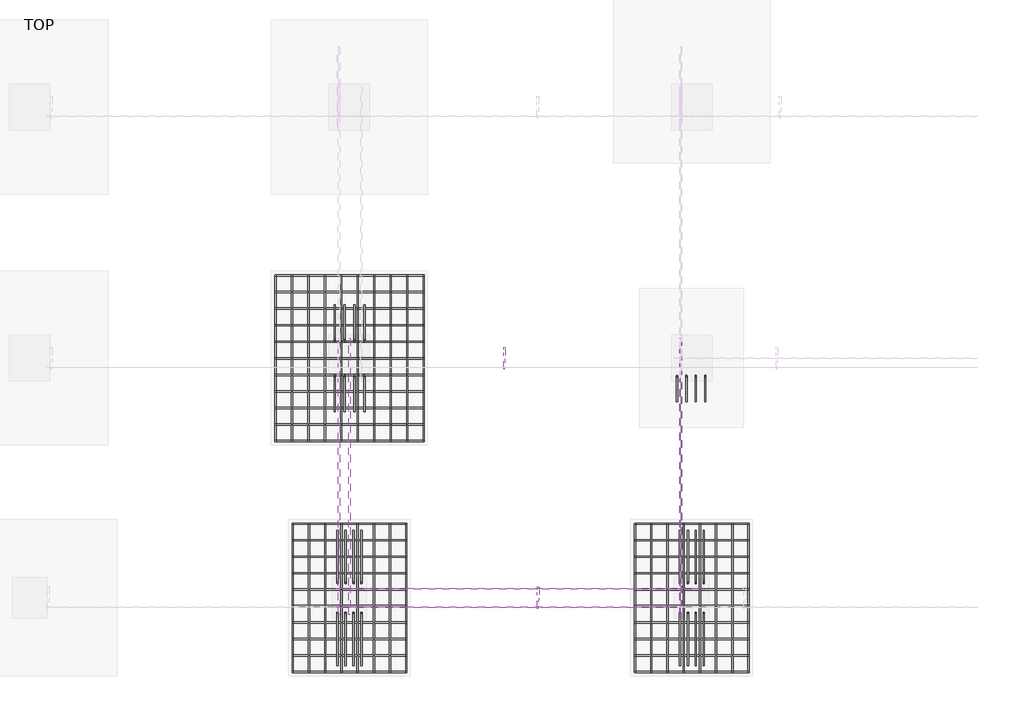
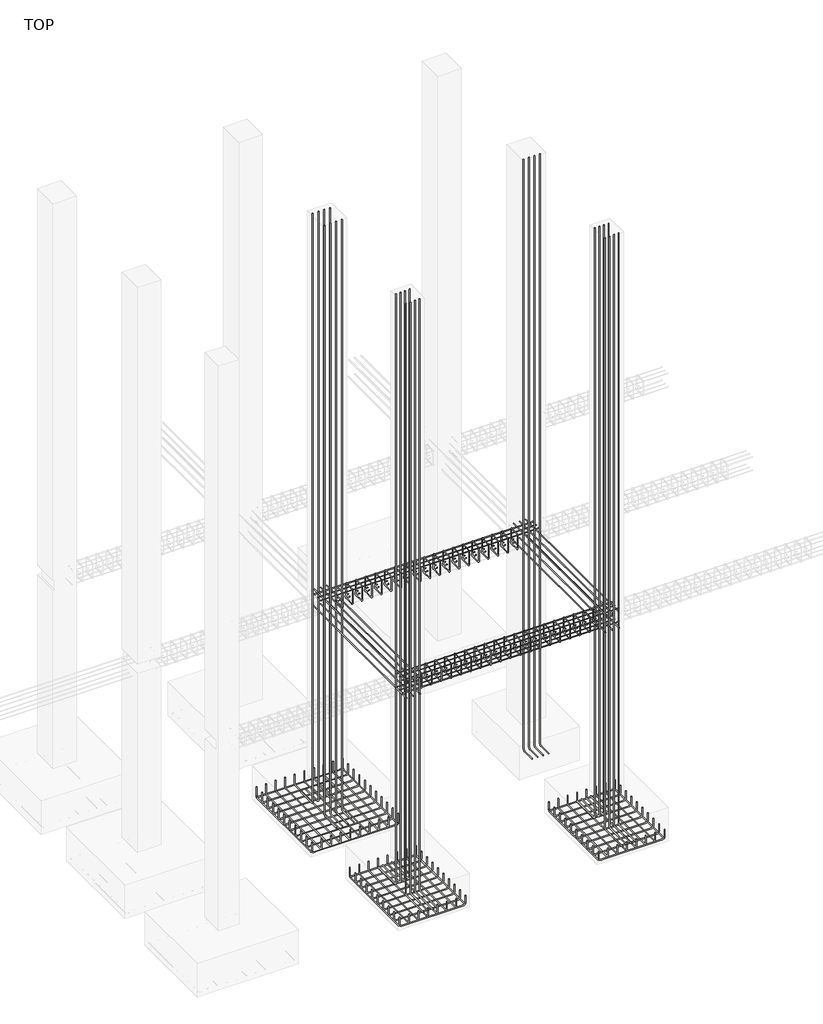
# One storey, part 5 of 8: 22 reinforcing bars.
"""IFC4 building model written with IfcOpenShell, lengths in millimetres."""

from ifc_helpers import new_model, si_unit, point, frame, origin, place, context, project, spatial, polyline, circle_curve, trimmed, segment, composite_curve, source, transform, mapped, element, save
from ifc_brep_helpers import swept_disk

model = new_model("IFC4")

# Units and contexts
model_context = context("Model", 3, world=origin())
ifc_project = project(units=[si_unit("LENGTHUNIT", "METRE", prefix="MILLI")], contexts=[model_context])

# Site, building, storey
site = spatial("IfcSite", under=ifc_project)
building = spatial("IfcBuilding", under=site)
storey = spatial("IfcBuildingStorey", under=building, Name="TOP", Elevation=0.0)

# Reinforcing bars
placement = place(None, origin())
reinforcing_bar_shape = source(origin(), model_context, "Body", "SolidModel", [
    swept_disk(composite_curve([segment(polyline([(3952.1028571, 3065.9815576, 8968.464), (3952.1028571, 3065.9815576, -415.886)]), True, "CONTINUOUS"), segment(trimmed(circle_curve(frame((3952.1028571, 3035.9815576, -415.886), z_axis=(-1.0, 0.0, 0.0), x_axis=(0.0, 30.0, 0.0)), 30.0), [point((3952.1028571, 3065.9815576, -415.886))], [point((3952.1028571, 3035.9815576, -445.886))], True, "CARTESIAN"), True, "CONTINUOUS"), segment(polyline([(3952.1028571, 3035.9815576, -445.886), (3952.1028571, 2842.0307576, -445.886)]), True, "CONTINUOUS")], self_intersect=False), 6.0),
])
element("IfcReinforcingBar", 1, at=placement, inside=storey, context=model_context, shape_type="MappedRepresentation", body=[
    mapped(reinforcing_bar_shape, transform((0.0, 0.0, 0.0), x_axis=(1.0, 0.0, 0.0), y_axis=(0.0, 1.0, 0.0), z_axis=(0.0, 0.0, 1.0))),
    mapped(reinforcing_bar_shape, transform((-82.2899057, 0.0, 0.0), x_axis=(1.0, 0.0, 0.0), y_axis=(0.0, 1.0, 0.0), z_axis=(0.0, 0.0, 1.0))),
    mapped(reinforcing_bar_shape, transform((-164.5798115, 0.0, 0.0), x_axis=(1.0, 0.0, 0.0), y_axis=(0.0, 1.0, 0.0), z_axis=(0.0, 0.0, 1.0))),
    mapped(reinforcing_bar_shape, transform((-246.8697172, 0.0, 0.0), x_axis=(1.0, 0.0, 0.0), y_axis=(0.0, 1.0, 0.0), z_axis=(0.0, 0.0, 1.0))),
])
reinforcing_bar_2_shape = source(origin(), model_context, "Body", "SolidModel", [
    swept_disk(composite_curve([segment(polyline([(730.6839399, 1250.9815576, 8968.464), (730.6839399, 1250.9815576, -409.536)]), True, "CONTINUOUS"), segment(trimmed(circle_curve(frame((730.6839399, 1280.9815576, -409.536), z_axis=(1.0, 0.0, 0.0), x_axis=(0.0, -30.0, 0.0)), 30.0), [point((730.6839399, 1250.9815576, -409.536))], [point((730.6839399, 1280.9815576, -439.536))], True, "CARTESIAN"), True, "CONTINUOUS"), segment(polyline([(730.6839399, 1280.9815576, -439.536), (730.6839399, 1716.1815576, -439.536)]), True, "CONTINUOUS")], self_intersect=False), 6.0),
])
element("IfcReinforcingBar", 2, at=placement, inside=storey, context=model_context, shape_type="MappedRepresentation", body=[
    mapped(reinforcing_bar_2_shape, transform((0.0, 0.0, 0.0), x_axis=(1.0, 0.0, 0.0), y_axis=(0.0, 1.0, 0.0), z_axis=(0.0, 0.0, 1.0))),
    mapped(reinforcing_bar_2_shape, transform((69.6, 0.0, 0.0), x_axis=(1.0, 0.0, 0.0), y_axis=(0.0, 1.0, 0.0), z_axis=(0.0, 0.0, 1.0))),
    mapped(reinforcing_bar_2_shape, transform((139.2, 0.0, 0.0), x_axis=(1.0, 0.0, 0.0), y_axis=(0.0, 1.0, 0.0), z_axis=(0.0, 0.0, 1.0))),
    mapped(reinforcing_bar_2_shape, transform((208.8, 0.0, 0.0), x_axis=(1.0, 0.0, 0.0), y_axis=(0.0, 1.0, 0.0), z_axis=(0.0, 0.0, 1.0))),
])
reinforcing_bar_3_shape = source(origin(), model_context, "Body", "SolidModel", [
    swept_disk(composite_curve([segment(polyline([(939.4839399, 991.2799576, 8968.464), (939.4839399, 991.2799576, -415.886)]), True, "CONTINUOUS"), segment(trimmed(circle_curve(frame((939.4839399, 961.2799576, -415.886), z_axis=(-1.0, 0.0, 0.0), x_axis=(0.0, 30.0, 0.0)), 30.0), [point((939.4839399, 991.2799576, -415.886))], [point((939.4839399, 961.2799576, -445.886))], True, "CARTESIAN"), True, "CONTINUOUS"), segment(polyline([(939.4839399, 961.2799576, -445.886), (939.4839399, 526.0799576, -445.886)]), True, "CONTINUOUS")], self_intersect=False), 6.0),
])
element("IfcReinforcingBar", 3, at=placement, inside=storey, context=model_context, shape_type="MappedRepresentation", body=[
    mapped(reinforcing_bar_3_shape, transform((0.0, 0.0, 0.0), x_axis=(1.0, 0.0, 0.0), y_axis=(0.0, 1.0, 0.0), z_axis=(0.0, 0.0, 1.0))),
    mapped(reinforcing_bar_3_shape, transform((-69.6, 0.0, 0.0), x_axis=(1.0, 0.0, 0.0), y_axis=(0.0, 1.0, 0.0), z_axis=(0.0, 0.0, 1.0))),
    mapped(reinforcing_bar_3_shape, transform((-139.2, 0.0, 0.0), x_axis=(1.0, 0.0, 0.0), y_axis=(0.0, 1.0, 0.0), z_axis=(0.0, 0.0, 1.0))),
    mapped(reinforcing_bar_3_shape, transform((-208.8, 0.0, 0.0), x_axis=(1.0, 0.0, 0.0), y_axis=(0.0, 1.0, 0.0), z_axis=(0.0, 0.0, 1.0))),
])
reinforcing_bar_4_shape = source(origin(), model_context, "Body", "SolidModel", [
    swept_disk(composite_curve([segment(polyline([(3730.6839399, 1250.9815576, 8968.464), (3730.6839399, 1250.9815576, -409.536)]), True, "CONTINUOUS"), segment(trimmed(circle_curve(frame((3730.6839399, 1280.9815576, -409.536), z_axis=(1.0, 0.0, 0.0), x_axis=(0.0, -30.0, 0.0)), 30.0), [point((3730.6839399, 1250.9815576, -409.536))], [point((3730.6839399, 1280.9815576, -439.536))], True, "CARTESIAN"), True, "CONTINUOUS"), segment(polyline([(3730.6839399, 1280.9815576, -439.536), (3730.6839399, 1716.1815576, -439.536)]), True, "CONTINUOUS")], self_intersect=False), 6.0),
])
element("IfcReinforcingBar", 4, at=placement, inside=storey, context=model_context, shape_type="MappedRepresentation", body=[
    mapped(reinforcing_bar_4_shape, transform((0.0, 0.0, 0.0), x_axis=(1.0, 0.0, 0.0), y_axis=(0.0, 1.0, 0.0), z_axis=(0.0, 0.0, 1.0))),
    mapped(reinforcing_bar_4_shape, transform((69.6, 0.0, 0.0), x_axis=(1.0, 0.0, 0.0), y_axis=(0.0, 1.0, 0.0), z_axis=(0.0, 0.0, 1.0))),
    mapped(reinforcing_bar_4_shape, transform((139.2, 0.0, 0.0), x_axis=(1.0, 0.0, 0.0), y_axis=(0.0, 1.0, 0.0), z_axis=(0.0, 0.0, 1.0))),
    mapped(reinforcing_bar_4_shape, transform((208.8, 0.0, 0.0), x_axis=(1.0, 0.0, 0.0), y_axis=(0.0, 1.0, 0.0), z_axis=(0.0, 0.0, 1.0))),
])
reinforcing_bar_5_shape = source(origin(), model_context, "Body", "SolidModel", [
    swept_disk(composite_curve([segment(polyline([(3939.4839399, 991.2799576, 8968.464), (3939.4839399, 991.2799576, -415.886)]), True, "CONTINUOUS"), segment(trimmed(circle_curve(frame((3939.4839399, 961.2799576, -415.886), z_axis=(-1.0, 0.0, 0.0), x_axis=(0.0, 30.0, 0.0)), 30.0), [point((3939.4839399, 991.2799576, -415.886))], [point((3939.4839399, 961.2799576, -445.886))], True, "CARTESIAN"), True, "CONTINUOUS"), segment(polyline([(3939.4839399, 961.2799576, -445.886), (3939.4839399, 526.0799576, -445.886)]), True, "CONTINUOUS")], self_intersect=False), 6.0),
])
element("IfcReinforcingBar", 5, at=placement, inside=storey, context=model_context, shape_type="MappedRepresentation", body=[
    mapped(reinforcing_bar_5_shape, transform((0.0, 0.0, 0.0), x_axis=(1.0, 0.0, 0.0), y_axis=(0.0, 1.0, 0.0), z_axis=(0.0, 0.0, 1.0))),
    mapped(reinforcing_bar_5_shape, transform((-69.6, 0.0, 0.0), x_axis=(1.0, 0.0, 0.0), y_axis=(0.0, 1.0, 0.0), z_axis=(0.0, 0.0, 1.0))),
    mapped(reinforcing_bar_5_shape, transform((-139.2, 0.0, 0.0), x_axis=(1.0, 0.0, 0.0), y_axis=(0.0, 1.0, 0.0), z_axis=(0.0, 0.0, 1.0))),
    mapped(reinforcing_bar_5_shape, transform((-208.8, 0.0, 0.0), x_axis=(1.0, 0.0, 0.0), y_axis=(0.0, 1.0, 0.0), z_axis=(0.0, 0.0, 1.0))),
])
reinforcing_bar_6_shape = source(origin(), model_context, "Body", "SolidModel", [
    swept_disk(composite_curve([segment(polyline([(1332.4839399, 1770.9307576, -351.0), (1332.4839399, 1770.9307576, -467.4)]), True, "CONTINUOUS"), segment(trimmed(circle_curve(frame((1332.4839399, 1740.9307576, -467.4), z_axis=(-1.0, 0.0, 0.0), x_axis=(0.0, 30.0, 0.0)), 30.0), [point((1332.4839399, 1770.9307576, -467.4))], [point((1332.4839399, 1740.9307576, -497.4))], True, "CARTESIAN"), True, "CONTINUOUS"), segment(polyline([(1332.4839399, 1740.9307576, -497.4), (1332.4839399, 501.3307576, -497.4)]), True, "CONTINUOUS"), segment(trimmed(circle_curve(frame((1332.4839399, 501.3307576, -467.4), z_axis=(-1.0, 0.0, 0.0), x_axis=(0.0, 0.0, -30.0)), 30.0), [point((1332.4839399, 501.3307576, -497.4))], [point((1332.4839399, 471.3307576, -467.4))], True, "CARTESIAN"), True, "CONTINUOUS"), segment(polyline([(1332.4839399, 471.3307576, -467.4), (1332.4839399, 471.3307576, -351.0)]), True, "CONTINUOUS")], self_intersect=False), 6.0),
])
element("IfcReinforcingBar", 6, at=placement, inside=storey, context=model_context, shape_type="MappedRepresentation", body=[
    mapped(reinforcing_bar_6_shape, transform((0.0, 0.0, 0.0), x_axis=(1.0, 0.0, 0.0), y_axis=(0.0, 1.0, 0.0), z_axis=(0.0, 0.0, 1.0))),
    mapped(reinforcing_bar_6_shape, transform((-142.1142857, 0.0, 0.0), x_axis=(1.0, 0.0, 0.0), y_axis=(0.0, 1.0, 0.0), z_axis=(0.0, 0.0, 1.0))),
    mapped(reinforcing_bar_6_shape, transform((-284.2285714, 0.0, 0.0), x_axis=(1.0, 0.0, 0.0), y_axis=(0.0, 1.0, 0.0), z_axis=(0.0, 0.0, 1.0))),
    mapped(reinforcing_bar_6_shape, transform((-426.3428571, 0.0, 0.0), x_axis=(1.0, 0.0, 0.0), y_axis=(0.0, 1.0, 0.0), z_axis=(0.0, 0.0, 1.0))),
    mapped(reinforcing_bar_6_shape, transform((-568.4571429, 0.0, 0.0), x_axis=(1.0, 0.0, 0.0), y_axis=(0.0, 1.0, 0.0), z_axis=(0.0, 0.0, 1.0))),
    mapped(reinforcing_bar_6_shape, transform((-710.5714286, 0.0, 0.0), x_axis=(1.0, 0.0, 0.0), y_axis=(0.0, 1.0, 0.0), z_axis=(0.0, 0.0, 1.0))),
    mapped(reinforcing_bar_6_shape, transform((-852.6857143, 0.0, 0.0), x_axis=(1.0, 0.0, 0.0), y_axis=(0.0, 1.0, 0.0), z_axis=(0.0, 0.0, 1.0))),
    mapped(reinforcing_bar_6_shape, transform((-994.8, 0.0, 0.0), x_axis=(1.0, 0.0, 0.0), y_axis=(0.0, 1.0, 0.0), z_axis=(0.0, 0.0, 1.0))),
])
reinforcing_bar_7_shape = source(origin(), model_context, "Body", "SolidModel", [
    swept_disk(composite_curve([segment(polyline([(337.6839399, 1770.9307576, -351.0), (337.6839399, 1770.9307576, -467.4)]), True, "CONTINUOUS"), segment(trimmed(circle_curve(frame((367.6839399, 1770.9307576, -467.4), z_axis=(0.0, -1.0, 0.0), x_axis=(-30.0, 0.0, 0.0)), 30.0), [point((337.6839399, 1770.9307576, -467.4))], [point((367.6839399, 1770.9307576, -497.4))], True, "CARTESIAN"), True, "CONTINUOUS"), segment(polyline([(367.6839399, 1770.9307576, -497.4), (1302.4839399, 1770.9307576, -497.4)]), True, "CONTINUOUS"), segment(trimmed(circle_curve(frame((1302.4839399, 1770.9307576, -467.4), z_axis=(0.0, -1.0, 0.0), x_axis=(0.0, 0.0, -30.0)), 30.0), [point((1302.4839399, 1770.9307576, -497.4))], [point((1332.4839399, 1770.9307576, -467.4))], True, "CARTESIAN"), True, "CONTINUOUS"), segment(polyline([(1332.4839399, 1770.9307576, -467.4), (1332.4839399, 1770.9307576, -351.0)]), True, "CONTINUOUS")], self_intersect=False), 6.0),
])
element("IfcReinforcingBar", 7, at=placement, inside=storey, context=model_context, shape_type="MappedRepresentation", body=[
    mapped(reinforcing_bar_7_shape, transform((0.0, 0.0, 0.0), x_axis=(1.0, 0.0, 0.0), y_axis=(0.0, 1.0, 0.0), z_axis=(0.0, 0.0, 1.0))),
    mapped(reinforcing_bar_7_shape, transform((0.0, -144.4, 0.0), x_axis=(1.0, 0.0, 0.0), y_axis=(0.0, 1.0, 0.0), z_axis=(0.0, 0.0, 1.0))),
    mapped(reinforcing_bar_7_shape, transform((0.0, -288.8, 0.0), x_axis=(1.0, 0.0, 0.0), y_axis=(0.0, 1.0, 0.0), z_axis=(0.0, 0.0, 1.0))),
    mapped(reinforcing_bar_7_shape, transform((0.0, -433.2, 0.0), x_axis=(1.0, 0.0, 0.0), y_axis=(0.0, 1.0, 0.0), z_axis=(0.0, 0.0, 1.0))),
    mapped(reinforcing_bar_7_shape, transform((0.0, -577.6, 0.0), x_axis=(1.0, 0.0, 0.0), y_axis=(0.0, 1.0, 0.0), z_axis=(0.0, 0.0, 1.0))),
    mapped(reinforcing_bar_7_shape, transform((0.0, -722.0, 0.0), x_axis=(1.0, 0.0, 0.0), y_axis=(0.0, 1.0, 0.0), z_axis=(0.0, 0.0, 1.0))),
    mapped(reinforcing_bar_7_shape, transform((0.0, -866.4, 0.0), x_axis=(1.0, 0.0, 0.0), y_axis=(0.0, 1.0, 0.0), z_axis=(0.0, 0.0, 1.0))),
    mapped(reinforcing_bar_7_shape, transform((0.0, -1010.8, 0.0), x_axis=(1.0, 0.0, 0.0), y_axis=(0.0, 1.0, 0.0), z_axis=(0.0, 0.0, 1.0))),
    mapped(reinforcing_bar_7_shape, transform((0.0, -1155.2, 0.0), x_axis=(1.0, 0.0, 0.0), y_axis=(0.0, 1.0, 0.0), z_axis=(0.0, 0.0, 1.0))),
    mapped(reinforcing_bar_7_shape, transform((0.0, -1299.6, 0.0), x_axis=(1.0, 0.0, 0.0), y_axis=(0.0, 1.0, 0.0), z_axis=(0.0, 0.0, 1.0))),
])
reinforcing_bar_8_shape = source(origin(), model_context, "Body", "SolidModel", [
    swept_disk(composite_curve([segment(polyline([(4332.4839399, 1770.9307576, -351.0), (4332.4839399, 1770.9307576, -467.4)]), True, "CONTINUOUS"), segment(trimmed(circle_curve(frame((4332.4839399, 1740.9307576, -467.4), z_axis=(-1.0, 0.0, 0.0), x_axis=(0.0, 30.0, 0.0)), 30.0), [point((4332.4839399, 1770.9307576, -467.4))], [point((4332.4839399, 1740.9307576, -497.4))], True, "CARTESIAN"), True, "CONTINUOUS"), segment(polyline([(4332.4839399, 1740.9307576, -497.4), (4332.4839399, 501.3307576, -497.4)]), True, "CONTINUOUS"), segment(trimmed(circle_curve(frame((4332.4839399, 501.3307576, -467.4), z_axis=(-1.0, 0.0, 0.0), x_axis=(0.0, 0.0, -30.0)), 30.0), [point((4332.4839399, 501.3307576, -497.4))], [point((4332.4839399, 471.3307576, -467.4))], True, "CARTESIAN"), True, "CONTINUOUS"), segment(polyline([(4332.4839399, 471.3307576, -467.4), (4332.4839399, 471.3307576, -351.0)]), True, "CONTINUOUS")], self_intersect=False), 6.0),
])
element("IfcReinforcingBar", 8, at=placement, inside=storey, context=model_context, shape_type="MappedRepresentation", body=[
    mapped(reinforcing_bar_8_shape, transform((0.0, 0.0, 0.0), x_axis=(1.0, 0.0, 0.0), y_axis=(0.0, 1.0, 0.0), z_axis=(0.0, 0.0, 1.0))),
    mapped(reinforcing_bar_8_shape, transform((-142.1142857, 0.0, 0.0), x_axis=(1.0, 0.0, 0.0), y_axis=(0.0, 1.0, 0.0), z_axis=(0.0, 0.0, 1.0))),
    mapped(reinforcing_bar_8_shape, transform((-284.2285714, 0.0, 0.0), x_axis=(1.0, 0.0, 0.0), y_axis=(0.0, 1.0, 0.0), z_axis=(0.0, 0.0, 1.0))),
    mapped(reinforcing_bar_8_shape, transform((-426.3428571, 0.0, 0.0), x_axis=(1.0, 0.0, 0.0), y_axis=(0.0, 1.0, 0.0), z_axis=(0.0, 0.0, 1.0))),
    mapped(reinforcing_bar_8_shape, transform((-568.4571429, 0.0, 0.0), x_axis=(1.0, 0.0, 0.0), y_axis=(0.0, 1.0, 0.0), z_axis=(0.0, 0.0, 1.0))),
    mapped(reinforcing_bar_8_shape, transform((-710.5714286, 0.0, 0.0), x_axis=(1.0, 0.0, 0.0), y_axis=(0.0, 1.0, 0.0), z_axis=(0.0, 0.0, 1.0))),
    mapped(reinforcing_bar_8_shape, transform((-852.6857143, 0.0, 0.0), x_axis=(1.0, 0.0, 0.0), y_axis=(0.0, 1.0, 0.0), z_axis=(0.0, 0.0, 1.0))),
    mapped(reinforcing_bar_8_shape, transform((-994.8, 0.0, 0.0), x_axis=(1.0, 0.0, 0.0), y_axis=(0.0, 1.0, 0.0), z_axis=(0.0, 0.0, 1.0))),
])
reinforcing_bar_9_shape = source(origin(), model_context, "Body", "SolidModel", [
    swept_disk(composite_curve([segment(polyline([(3337.6839399, 1770.9307576, -351.0), (3337.6839399, 1770.9307576, -467.4)]), True, "CONTINUOUS"), segment(trimmed(circle_curve(frame((3367.6839399, 1770.9307576, -467.4), z_axis=(0.0, -1.0, 0.0), x_axis=(-30.0, 0.0, 0.0)), 30.0), [point((3337.6839399, 1770.9307576, -467.4))], [point((3367.6839399, 1770.9307576, -497.4))], True, "CARTESIAN"), True, "CONTINUOUS"), segment(polyline([(3367.6839399, 1770.9307576, -497.4), (4302.4839399, 1770.9307576, -497.4)]), True, "CONTINUOUS"), segment(trimmed(circle_curve(frame((4302.4839399, 1770.9307576, -467.4), z_axis=(0.0, -1.0, 0.0), x_axis=(0.0, 0.0, -30.0)), 30.0), [point((4302.4839399, 1770.9307576, -497.4))], [point((4332.4839399, 1770.9307576, -467.4))], True, "CARTESIAN"), True, "CONTINUOUS"), segment(polyline([(4332.4839399, 1770.9307576, -467.4), (4332.4839399, 1770.9307576, -351.0)]), True, "CONTINUOUS")], self_intersect=False), 6.0),
])
element("IfcReinforcingBar", 9, at=placement, inside=storey, context=model_context, shape_type="MappedRepresentation", body=[
    mapped(reinforcing_bar_9_shape, transform((0.0, 0.0, 0.0), x_axis=(1.0, 0.0, 0.0), y_axis=(0.0, 1.0, 0.0), z_axis=(0.0, 0.0, 1.0))),
    mapped(reinforcing_bar_9_shape, transform((0.0, -144.4, 0.0), x_axis=(1.0, 0.0, 0.0), y_axis=(0.0, 1.0, 0.0), z_axis=(0.0, 0.0, 1.0))),
    mapped(reinforcing_bar_9_shape, transform((0.0, -288.8, 0.0), x_axis=(1.0, 0.0, 0.0), y_axis=(0.0, 1.0, 0.0), z_axis=(0.0, 0.0, 1.0))),
    mapped(reinforcing_bar_9_shape, transform((0.0, -433.2, 0.0), x_axis=(1.0, 0.0, 0.0), y_axis=(0.0, 1.0, 0.0), z_axis=(0.0, 0.0, 1.0))),
    mapped(reinforcing_bar_9_shape, transform((0.0, -577.6, 0.0), x_axis=(1.0, 0.0, 0.0), y_axis=(0.0, 1.0, 0.0), z_axis=(0.0, 0.0, 1.0))),
    mapped(reinforcing_bar_9_shape, transform((0.0, -722.0, 0.0), x_axis=(1.0, 0.0, 0.0), y_axis=(0.0, 1.0, 0.0), z_axis=(0.0, 0.0, 1.0))),
    mapped(reinforcing_bar_9_shape, transform((0.0, -866.4, 0.0), x_axis=(1.0, 0.0, 0.0), y_axis=(0.0, 1.0, 0.0), z_axis=(0.0, 0.0, 1.0))),
    mapped(reinforcing_bar_9_shape, transform((0.0, -1010.8, 0.0), x_axis=(1.0, 0.0, 0.0), y_axis=(0.0, 1.0, 0.0), z_axis=(0.0, 0.0, 1.0))),
    mapped(reinforcing_bar_9_shape, transform((0.0, -1155.2, 0.0), x_axis=(1.0, 0.0, 0.0), y_axis=(0.0, 1.0, 0.0), z_axis=(0.0, 0.0, 1.0))),
    mapped(reinforcing_bar_9_shape, transform((0.0, -1299.6, 0.0), x_axis=(1.0, 0.0, 0.0), y_axis=(0.0, 1.0, 0.0), z_axis=(0.0, 0.0, 1.0))),
])
reinforcing_bar_10_shape = source(origin(), model_context, "Body", "SolidModel", [
    swept_disk(composite_curve([segment(polyline([(705.2331399, 3376.2799576, 8968.464), (705.2331399, 3376.2799576, -403.186)]), True, "CONTINUOUS"), segment(trimmed(circle_curve(frame((705.2331399, 3406.2799576, -403.186), z_axis=(1.0, 0.0, 0.0), x_axis=(0.0, -30.0, 0.0)), 30.0), [point((705.2331399, 3376.2799576, -403.186))], [point((705.2331399, 3406.2799576, -433.186))], True, "CARTESIAN"), True, "CONTINUOUS"), segment(polyline([(705.2331399, 3406.2799576, -433.186), (705.2331399, 3689.0799576, -433.186)]), True, "CONTINUOUS")], self_intersect=False), 6.0),
])
element("IfcReinforcingBar", 10, at=placement, inside=storey, context=model_context, shape_type="MappedRepresentation", body=[
    mapped(reinforcing_bar_10_shape, transform((0.0, 0.0, 0.0), x_axis=(1.0, 0.0, 0.0), y_axis=(0.0, 1.0, 0.0), z_axis=(0.0, 0.0, 1.0))),
    mapped(reinforcing_bar_10_shape, transform((86.5672, 0.0, 0.0), x_axis=(1.0, 0.0, 0.0), y_axis=(0.0, 1.0, 0.0), z_axis=(0.0, 0.0, 1.0))),
    mapped(reinforcing_bar_10_shape, transform((173.1344, 0.0, 0.0), x_axis=(1.0, 0.0, 0.0), y_axis=(0.0, 1.0, 0.0), z_axis=(0.0, 0.0, 1.0))),
    mapped(reinforcing_bar_10_shape, transform((259.7016, 0.0, 0.0), x_axis=(1.0, 0.0, 0.0), y_axis=(0.0, 1.0, 0.0), z_axis=(0.0, 0.0, 1.0))),
])
reinforcing_bar_11_shape = source(origin(), model_context, "Body", "SolidModel", [
    swept_disk(composite_curve([segment(polyline([(964.9347399, 3065.9815576, 8968.464), (964.9347399, 3065.9815576, -409.536)]), True, "CONTINUOUS"), segment(trimmed(circle_curve(frame((964.9347399, 3035.9815576, -409.536), z_axis=(-1.0, 0.0, 0.0), x_axis=(0.0, 30.0, 0.0)), 30.0), [point((964.9347399, 3065.9815576, -409.536))], [point((964.9347399, 3035.9815576, -439.536))], True, "CARTESIAN"), True, "CONTINUOUS"), segment(polyline([(964.9347399, 3035.9815576, -439.536), (964.9347399, 2753.1815576, -439.536)]), True, "CONTINUOUS")], self_intersect=False), 6.0),
])
element("IfcReinforcingBar", 11, at=placement, inside=storey, context=model_context, shape_type="MappedRepresentation", body=[
    mapped(reinforcing_bar_11_shape, transform((0.0, 0.0, 0.0), x_axis=(1.0, 0.0, 0.0), y_axis=(0.0, 1.0, 0.0), z_axis=(0.0, 0.0, 1.0))),
    mapped(reinforcing_bar_11_shape, transform((-86.5672, 0.0, 0.0), x_axis=(1.0, 0.0, 0.0), y_axis=(0.0, 1.0, 0.0), z_axis=(0.0, 0.0, 1.0))),
    mapped(reinforcing_bar_11_shape, transform((-173.1344, 0.0, 0.0), x_axis=(1.0, 0.0, 0.0), y_axis=(0.0, 1.0, 0.0), z_axis=(0.0, 0.0, 1.0))),
    mapped(reinforcing_bar_11_shape, transform((-259.7016, 0.0, 0.0), x_axis=(1.0, 0.0, 0.0), y_axis=(0.0, 1.0, 0.0), z_axis=(0.0, 0.0, 1.0))),
])
reinforcing_bar_12_shape = source(origin(), model_context, "Body", "SolidModel", [
    swept_disk(composite_curve([segment(polyline([(185.2839399, 3947.1307576, -331.0), (185.2839399, 3947.1307576, -467.4)]), True, "CONTINUOUS"), segment(trimmed(circle_curve(frame((215.2839399, 3947.1307576, -467.4), z_axis=(0.0, -1.0, 0.0), x_axis=(-30.0, 0.0, 0.0)), 30.0), [point((185.2839399, 3947.1307576, -467.4))], [point((215.2839399, 3947.1307576, -497.4))], True, "CARTESIAN"), True, "CONTINUOUS"), segment(polyline([(215.2839399, 3947.1307576, -497.4), (1454.8839399, 3947.1307576, -497.4)]), True, "CONTINUOUS"), segment(trimmed(circle_curve(frame((1454.8839399, 3947.1307576, -467.4), z_axis=(0.0, -1.0, 0.0), x_axis=(0.0, 0.0, -30.0)), 30.0), [point((1454.8839399, 3947.1307576, -497.4))], [point((1484.8839399, 3947.1307576, -467.4))], True, "CARTESIAN"), True, "CONTINUOUS"), segment(polyline([(1484.8839399, 3947.1307576, -467.4), (1484.8839399, 3947.1307576, -331.0)]), True, "CONTINUOUS")], self_intersect=False), 6.0),
])
element("IfcReinforcingBar", 12, at=placement, inside=storey, context=model_context, shape_type="MappedRepresentation", body=[
    mapped(reinforcing_bar_12_shape, transform((0.0, 0.0, 0.0), x_axis=(1.0, 0.0, 0.0), y_axis=(0.0, 1.0, 0.0), z_axis=(0.0, 0.0, 1.0))),
    mapped(reinforcing_bar_12_shape, transform((0.0, -145.2, 0.0), x_axis=(1.0, 0.0, 0.0), y_axis=(0.0, 1.0, 0.0), z_axis=(0.0, 0.0, 1.0))),
    mapped(reinforcing_bar_12_shape, transform((0.0, -290.4, 0.0), x_axis=(1.0, 0.0, 0.0), y_axis=(0.0, 1.0, 0.0), z_axis=(0.0, 0.0, 1.0))),
    mapped(reinforcing_bar_12_shape, transform((0.0, -435.6, 0.0), x_axis=(1.0, 0.0, 0.0), y_axis=(0.0, 1.0, 0.0), z_axis=(0.0, 0.0, 1.0))),
    mapped(reinforcing_bar_12_shape, transform((0.0, -580.8, 0.0), x_axis=(1.0, 0.0, 0.0), y_axis=(0.0, 1.0, 0.0), z_axis=(0.0, 0.0, 1.0))),
    mapped(reinforcing_bar_12_shape, transform((0.0, -726.0, 0.0), x_axis=(1.0, 0.0, 0.0), y_axis=(0.0, 1.0, 0.0), z_axis=(0.0, 0.0, 1.0))),
    mapped(reinforcing_bar_12_shape, transform((0.0, -871.2, 0.0), x_axis=(1.0, 0.0, 0.0), y_axis=(0.0, 1.0, 0.0), z_axis=(0.0, 0.0, 1.0))),
    mapped(reinforcing_bar_12_shape, transform((0.0, -1016.4, 0.0), x_axis=(1.0, 0.0, 0.0), y_axis=(0.0, 1.0, 0.0), z_axis=(0.0, 0.0, 1.0))),
    mapped(reinforcing_bar_12_shape, transform((0.0, -1161.6, 0.0), x_axis=(1.0, 0.0, 0.0), y_axis=(0.0, 1.0, 0.0), z_axis=(0.0, 0.0, 1.0))),
    mapped(reinforcing_bar_12_shape, transform((0.0, -1306.8, 0.0), x_axis=(1.0, 0.0, 0.0), y_axis=(0.0, 1.0, 0.0), z_axis=(0.0, 0.0, 1.0))),
    mapped(reinforcing_bar_12_shape, transform((0.0, -1452.0, 0.0), x_axis=(1.0, 0.0, 0.0), y_axis=(0.0, 1.0, 0.0), z_axis=(0.0, 0.0, 1.0))),
])
reinforcing_bar_13_shape = source(origin(), model_context, "Body", "SolidModel", [
    swept_disk(composite_curve([segment(polyline([(185.2839399, 2495.1307576, -331.0), (185.2839399, 2495.1307576, -467.4)]), True, "CONTINUOUS"), segment(trimmed(circle_curve(frame((185.2839399, 2525.1307576, -467.4), z_axis=(1.0, 0.0, 0.0), x_axis=(0.0, -30.0, 0.0)), 30.0), [point((185.2839399, 2495.1307576, -467.4))], [point((185.2839399, 2525.1307576, -497.4))], True, "CARTESIAN"), True, "CONTINUOUS"), segment(polyline([(185.2839399, 2525.1307576, -497.4), (185.2839399, 3917.1307576, -497.4)]), True, "CONTINUOUS"), segment(trimmed(circle_curve(frame((185.2839399, 3917.1307576, -467.4), z_axis=(1.0, 0.0, 0.0), x_axis=(0.0, 0.0, -30.0)), 30.0), [point((185.2839399, 3917.1307576, -497.4))], [point((185.2839399, 3947.1307576, -467.4))], True, "CARTESIAN"), True, "CONTINUOUS"), segment(polyline([(185.2839399, 3947.1307576, -467.4), (185.2839399, 3947.1307576, -331.0)]), True, "CONTINUOUS")], self_intersect=False), 6.0),
])
element("IfcReinforcingBar", 13, at=placement, inside=storey, context=model_context, shape_type="MappedRepresentation", body=[
    mapped(reinforcing_bar_13_shape, transform((0.0, 0.0, 0.0), x_axis=(1.0, 0.0, 0.0), y_axis=(0.0, 1.0, 0.0), z_axis=(0.0, 0.0, 1.0))),
    mapped(reinforcing_bar_13_shape, transform((144.4, 0.0, 0.0), x_axis=(1.0, 0.0, 0.0), y_axis=(0.0, 1.0, 0.0), z_axis=(0.0, 0.0, 1.0))),
    mapped(reinforcing_bar_13_shape, transform((288.8, 0.0, 0.0), x_axis=(1.0, 0.0, 0.0), y_axis=(0.0, 1.0, 0.0), z_axis=(0.0, 0.0, 1.0))),
    mapped(reinforcing_bar_13_shape, transform((433.2, 0.0, 0.0), x_axis=(1.0, 0.0, 0.0), y_axis=(0.0, 1.0, 0.0), z_axis=(0.0, 0.0, 1.0))),
    mapped(reinforcing_bar_13_shape, transform((577.6, 0.0, 0.0), x_axis=(1.0, 0.0, 0.0), y_axis=(0.0, 1.0, 0.0), z_axis=(0.0, 0.0, 1.0))),
    mapped(reinforcing_bar_13_shape, transform((722.0, 0.0, 0.0), x_axis=(1.0, 0.0, 0.0), y_axis=(0.0, 1.0, 0.0), z_axis=(0.0, 0.0, 1.0))),
    mapped(reinforcing_bar_13_shape, transform((866.4, 0.0, 0.0), x_axis=(1.0, 0.0, 0.0), y_axis=(0.0, 1.0, 0.0), z_axis=(0.0, 0.0, 1.0))),
    mapped(reinforcing_bar_13_shape, transform((1010.8, 0.0, 0.0), x_axis=(1.0, 0.0, 0.0), y_axis=(0.0, 1.0, 0.0), z_axis=(0.0, 0.0, 1.0))),
    mapped(reinforcing_bar_13_shape, transform((1155.2, 0.0, 0.0), x_axis=(1.0, 0.0, 0.0), y_axis=(0.0, 1.0, 0.0), z_axis=(0.0, 0.0, 1.0))),
    mapped(reinforcing_bar_13_shape, transform((1299.6, 0.0, 0.0), x_axis=(1.0, 0.0, 0.0), y_axis=(0.0, 1.0, 0.0), z_axis=(0.0, 0.0, 1.0))),
])
reinforcing_bar_14_shape = source(origin(), model_context, "Body", "SolidModel", [
    swept_disk(composite_curve([segment(polyline([(732.0773382, 3394.2799576, 2693.6917983), (732.0773382, 973.2799576, 2693.6917983)]), True, "CONTINUOUS")], self_intersect=False), 5.0),
])
element("IfcReinforcingBar", 14, at=placement, inside=storey, context=model_context, shape_type="MappedRepresentation", body=[
    mapped(reinforcing_bar_14_shape, transform((0.0, 0.0, 0.0), x_axis=(1.0, 0.0, 0.0), y_axis=(0.0, 1.0, 0.0), z_axis=(0.0, 0.0, 1.0))),
    mapped(reinforcing_bar_14_shape, transform((103.0066017, 0.0, 0.0), x_axis=(1.0, 0.0, 0.0), y_axis=(0.0, 1.0, 0.0), z_axis=(0.0, 0.0, 1.0))),
    mapped(reinforcing_bar_14_shape, transform((206.0132034, 0.0, 0.0), x_axis=(1.0, 0.0, 0.0), y_axis=(0.0, 1.0, 0.0), z_axis=(0.0, 0.0, 1.0))),
])
reinforcing_bar_15_shape = source(origin(), model_context, "Body", "SolidModel", [
    swept_disk(composite_curve([segment(polyline([(742.6839399, 973.2799576, 2955.0), (742.6839399, 3394.2799576, 2955.0)]), True, "CONTINUOUS")], self_intersect=False), 5.0),
])
element("IfcReinforcingBar", 15, at=placement, inside=storey, context=model_context, shape_type="MappedRepresentation", body=[
    mapped(reinforcing_bar_15_shape, transform((0.0, 0.0, 0.0), x_axis=(1.0, 0.0, 0.0), y_axis=(0.0, 1.0, 0.0), z_axis=(0.0, 0.0, 1.0))),
    mapped(reinforcing_bar_15_shape, transform((92.4, 0.0, 0.0), x_axis=(1.0, 0.0, 0.0), y_axis=(0.0, 1.0, 0.0), z_axis=(0.0, 0.0, 1.0))),
    mapped(reinforcing_bar_15_shape, transform((184.8, 0.0, 0.0), x_axis=(1.0, 0.0, 0.0), y_axis=(0.0, 1.0, 0.0), z_axis=(0.0, 0.0, 1.0))),
])
reinforcing_bar_16_shape = source(origin(), model_context, "Body", "SolidModel", [
    swept_disk(composite_curve([segment(polyline([(3732.0773382, 3394.2799576, 2693.6917983), (3732.0773382, 973.2799576, 2693.6917983)]), True, "CONTINUOUS")], self_intersect=False), 5.0),
])
element("IfcReinforcingBar", 16, at=placement, inside=storey, context=model_context, shape_type="MappedRepresentation", body=[
    mapped(reinforcing_bar_16_shape, transform((0.0, 0.0, 0.0), x_axis=(1.0, 0.0, 0.0), y_axis=(0.0, 1.0, 0.0), z_axis=(0.0, 0.0, 1.0))),
    mapped(reinforcing_bar_16_shape, transform((103.0066017, 0.0, 0.0), x_axis=(1.0, 0.0, 0.0), y_axis=(0.0, 1.0, 0.0), z_axis=(0.0, 0.0, 1.0))),
    mapped(reinforcing_bar_16_shape, transform((206.0132034, 0.0, 0.0), x_axis=(1.0, 0.0, 0.0), y_axis=(0.0, 1.0, 0.0), z_axis=(0.0, 0.0, 1.0))),
])
reinforcing_bar_17_shape = source(origin(), model_context, "Body", "SolidModel", [
    swept_disk(composite_curve([segment(polyline([(3742.6839399, 973.2799576, 2955.0), (3742.6839399, 3394.2799576, 2955.0)]), True, "CONTINUOUS")], self_intersect=False), 5.0),
])
element("IfcReinforcingBar", 17, at=placement, inside=storey, context=model_context, shape_type="MappedRepresentation", body=[
    mapped(reinforcing_bar_17_shape, transform((0.0, 0.0, 0.0), x_axis=(1.0, 0.0, 0.0), y_axis=(0.0, 1.0, 0.0), z_axis=(0.0, 0.0, 1.0))),
    mapped(reinforcing_bar_17_shape, transform((92.4, 0.0, 0.0), x_axis=(1.0, 0.0, 0.0), y_axis=(0.0, 1.0, 0.0), z_axis=(0.0, 0.0, 1.0))),
    mapped(reinforcing_bar_17_shape, transform((184.8, 0.0, 0.0), x_axis=(1.0, 0.0, 0.0), y_axis=(0.0, 1.0, 0.0), z_axis=(0.0, 0.0, 1.0))),
])
reinforcing_bar_18_shape = source(origin(), model_context, "Body", "SolidModel", [
    swept_disk(composite_curve([segment(polyline([(3678.2331399, 1143.8753761, 2827.6888527), (3678.2331399, 1208.2220932, 2763.3421356)]), True, "CONTINUOUS"), segment(trimmed(circle_curve(frame((3678.2331399, 1194.0799576, 2749.2), z_axis=(-1.0, 0.0, 0.0), x_axis=(0.0, 14.142135600000074, 14.142135600000074)), 20.0), [point((3678.2331399, 1208.2220932, 2763.3421356))], [point((3678.2331399, 1194.0799576, 2729.2))], True, "CARTESIAN"), True, "CONTINUOUS"), segment(polyline([(3678.2331399, 1194.0799576, 2729.2), (3678.2331399, 1048.1815576, 2729.2)]), True, "CONTINUOUS"), segment(trimmed(circle_curve(frame((3678.2331399, 1048.1815576, 2749.2), z_axis=(-1.0, 0.0, 0.0), x_axis=(0.0, 0.0, -20.0)), 20.0), [point((3678.2331399, 1048.1815576, 2729.2))], [point((3678.2331399, 1028.1815576, 2749.2))], True, "CARTESIAN"), True, "CONTINUOUS"), segment(polyline([(3678.2331399, 1028.1815576, 2749.2), (3678.2331399, 1028.1815576, 2946.0)]), True, "CONTINUOUS"), segment(trimmed(circle_curve(frame((3679.0930293, 1048.1630638, 2946.0), z_axis=(-0.9990753104108542, 0.04299446624224494, 0.0), x_axis=(-0.8598894000001565, -19.981506200000013, 0.0)), 20.0), [point((3678.2331399, 1028.1815576, 2946.0))], [point((3679.0930293, 1048.1630638, 2966.0))], True, "CARTESIAN"), True, "CONTINUOUS"), segment(polyline([(3679.0930293, 1048.1630638, 2966.0), (3685.3732506, 1194.0984514, 2966.0)]), True, "CONTINUOUS"), segment(trimmed(circle_curve(frame((3685.3732506, 1194.0984514, 2946.0), z_axis=(-0.9990753104108542, 0.04299446624224494, 0.0), x_axis=(0.0, 0.0, 20.0)), 20.0), [point((3685.3732506, 1194.0984514, 2966.0))], [point((3686.2331399, 1214.0799576, 2946.0))], True, "CARTESIAN"), True, "CONTINUOUS"), segment(polyline([(3686.2331399, 1214.0799576, 2946.0), (3686.2331399, 1214.0799576, 2749.2)]), True, "CONTINUOUS"), segment(trimmed(circle_curve(frame((3686.2331399, 1194.0799576, 2749.2), z_axis=(-1.0, 0.0, 0.0), x_axis=(0.0, 20.0, 0.0)), 20.0), [point((3686.2331399, 1214.0799576, 2749.2))], [point((3686.2331399, 1179.937822, 2735.0578644))], True, "CARTESIAN"), True, "CONTINUOUS"), segment(polyline([(3686.2331399, 1179.937822, 2735.0578644), (3686.2331399, 1115.5911049, 2799.4045815)]), True, "CONTINUOUS")], self_intersect=False), 4.0),
])
element("IfcReinforcingBar", 18, at=placement, inside=storey, context=model_context, shape_type="MappedRepresentation", body=[
    mapped(reinforcing_bar_18_shape, transform((0.0, 0.0, 0.0), x_axis=(1.0, 0.0, 0.0), y_axis=(0.0, 1.0, 0.0), z_axis=(0.0, 0.0, 1.0))),
    mapped(reinforcing_bar_18_shape, transform((-149.2638444, 0.0, 0.0), x_axis=(1.0, 0.0, 0.0), y_axis=(0.0, 1.0, 0.0), z_axis=(0.0, 0.0, 1.0))),
    mapped(reinforcing_bar_18_shape, transform((-298.5276889, 0.0, 0.0), x_axis=(1.0, 0.0, 0.0), y_axis=(0.0, 1.0, 0.0), z_axis=(0.0, 0.0, 1.0))),
    mapped(reinforcing_bar_18_shape, transform((-447.7915333, 0.0, 0.0), x_axis=(1.0, 0.0, 0.0), y_axis=(0.0, 1.0, 0.0), z_axis=(0.0, 0.0, 1.0))),
    mapped(reinforcing_bar_18_shape, transform((-597.0553778, 0.0, 0.0), x_axis=(1.0, 0.0, 0.0), y_axis=(0.0, 1.0, 0.0), z_axis=(0.0, 0.0, 1.0))),
    mapped(reinforcing_bar_18_shape, transform((-746.3192222, 0.0, 0.0), x_axis=(1.0, 0.0, 0.0), y_axis=(0.0, 1.0, 0.0), z_axis=(0.0, 0.0, 1.0))),
    mapped(reinforcing_bar_18_shape, transform((-895.5830667, 0.0, 0.0), x_axis=(1.0, 0.0, 0.0), y_axis=(0.0, 1.0, 0.0), z_axis=(0.0, 0.0, 1.0))),
    mapped(reinforcing_bar_18_shape, transform((-1044.8469111, 0.0, 0.0), x_axis=(1.0, 0.0, 0.0), y_axis=(0.0, 1.0, 0.0), z_axis=(0.0, 0.0, 1.0))),
    mapped(reinforcing_bar_18_shape, transform((-1194.1107556, 0.0, 0.0), x_axis=(1.0, 0.0, 0.0), y_axis=(0.0, 1.0, 0.0), z_axis=(0.0, 0.0, 1.0))),
    mapped(reinforcing_bar_18_shape, transform((-1343.3746, 0.0, 0.0), x_axis=(1.0, 0.0, 0.0), y_axis=(0.0, 1.0, 0.0), z_axis=(0.0, 0.0, 1.0))),
    mapped(reinforcing_bar_18_shape, transform((-1492.6384444, 0.0, 0.0), x_axis=(1.0, 0.0, 0.0), y_axis=(0.0, 1.0, 0.0), z_axis=(0.0, 0.0, 1.0))),
    mapped(reinforcing_bar_18_shape, transform((-1641.9022889, 0.0, 0.0), x_axis=(1.0, 0.0, 0.0), y_axis=(0.0, 1.0, 0.0), z_axis=(0.0, 0.0, 1.0))),
    mapped(reinforcing_bar_18_shape, transform((-1791.1661333, 0.0, 0.0), x_axis=(1.0, 0.0, 0.0), y_axis=(0.0, 1.0, 0.0), z_axis=(0.0, 0.0, 1.0))),
    mapped(reinforcing_bar_18_shape, transform((-1940.4299778, 0.0, 0.0), x_axis=(1.0, 0.0, 0.0), y_axis=(0.0, 1.0, 0.0), z_axis=(0.0, 0.0, 1.0))),
    mapped(reinforcing_bar_18_shape, transform((-2089.6938222, 0.0, 0.0), x_axis=(1.0, 0.0, 0.0), y_axis=(0.0, 1.0, 0.0), z_axis=(0.0, 0.0, 1.0))),
    mapped(reinforcing_bar_18_shape, transform((-2238.9576667, 0.0, 0.0), x_axis=(1.0, 0.0, 0.0), y_axis=(0.0, 1.0, 0.0), z_axis=(0.0, 0.0, 1.0))),
    mapped(reinforcing_bar_18_shape, transform((-2388.2215111, 0.0, 0.0), x_axis=(1.0, 0.0, 0.0), y_axis=(0.0, 1.0, 0.0), z_axis=(0.0, 0.0, 1.0))),
    mapped(reinforcing_bar_18_shape, transform((-2537.4853556, 0.0, 0.0), x_axis=(1.0, 0.0, 0.0), y_axis=(0.0, 1.0, 0.0), z_axis=(0.0, 0.0, 1.0))),
    mapped(reinforcing_bar_18_shape, transform((-2686.7492, 0.0, 0.0), x_axis=(1.0, 0.0, 0.0), y_axis=(0.0, 1.0, 0.0), z_axis=(0.0, 0.0, 1.0))),
])
reinforcing_bar_19_shape = source(origin(), model_context, "Body", "SolidModel", [
    swept_disk(composite_curve([segment(polyline([(3957.4839399, 1039.6962762, 2954.4852814), (712.6839399, 1039.6962762, 2954.4852814)]), True, "CONTINUOUS")], self_intersect=False), 4.0),
])
element("IfcReinforcingBar", 19, at=placement, inside=storey, context=model_context, shape_type="MappedRepresentation", body=[
    mapped(reinforcing_bar_19_shape, transform((0.0, 0.0, 0.0), x_axis=(1.0, 0.0, 0.0), y_axis=(0.0, 1.0, 0.0), z_axis=(0.0, 0.0, 1.0))),
    mapped(reinforcing_bar_19_shape, transform((0.0, 81.4344814, 0.0), x_axis=(1.0, 0.0, 0.0), y_axis=(0.0, 1.0, 0.0), z_axis=(0.0, 0.0, 1.0))),
    mapped(reinforcing_bar_19_shape, transform((0.0, 162.8689627, 0.0), x_axis=(1.0, 0.0, 0.0), y_axis=(0.0, 1.0, 0.0), z_axis=(0.0, 0.0, 1.0))),
])
reinforcing_bar_20_shape = source(origin(), model_context, "Body", "SolidModel", [
    swept_disk(composite_curve([segment(polyline([(3957.4839399, 1202.565239, 2740.7147186), (712.6839399, 1202.565239, 2740.7147186)]), True, "CONTINUOUS")], self_intersect=False), 4.0),
])
element("IfcReinforcingBar", 20, at=placement, inside=storey, context=model_context, shape_type="MappedRepresentation", body=[
    mapped(reinforcing_bar_20_shape, transform((0.0, 0.0, 0.0), x_axis=(1.0, 0.0, 0.0), y_axis=(0.0, 1.0, 0.0), z_axis=(0.0, 0.0, 1.0))),
    mapped(reinforcing_bar_20_shape, transform((0.0, -81.4344814, 0.0), x_axis=(1.0, 0.0, 0.0), y_axis=(0.0, 1.0, 0.0), z_axis=(0.0, 0.0, 1.0))),
    mapped(reinforcing_bar_20_shape, transform((0.0, -162.8689627, 0.0), x_axis=(1.0, 0.0, 0.0), y_axis=(0.0, 1.0, 0.0), z_axis=(0.0, 0.0, 1.0))),
])
reinforcing_bar_21_shape = source(origin(), model_context, "Body", "SolidModel", [
    swept_disk(composite_curve([segment(polyline([(3653.3823399, 3243.8753761, 2827.6888527), (3653.3823399, 3308.2220932, 2763.3421356)]), True, "CONTINUOUS"), segment(trimmed(circle_curve(frame((3653.3823399, 3294.0799576, 2749.2), z_axis=(-1.0, 0.0, 0.0), x_axis=(0.0, 14.142135600000074, 14.142135600000074)), 20.0), [point((3653.3823399, 3308.2220932, 2763.3421356))], [point((3653.3823399, 3294.0799576, 2729.2))], True, "CARTESIAN"), True, "CONTINUOUS"), segment(polyline([(3653.3823399, 3294.0799576, 2729.2), (3653.3823399, 3148.1815576, 2729.2)]), True, "CONTINUOUS"), segment(trimmed(circle_curve(frame((3653.3823399, 3148.1815576, 2749.2), z_axis=(-1.0, 0.0, 0.0), x_axis=(0.0, 0.0, -20.0)), 20.0), [point((3653.3823399, 3148.1815576, 2729.2))], [point((3653.3823399, 3128.1815576, 2749.2))], True, "CARTESIAN"), True, "CONTINUOUS"), segment(polyline([(3653.3823399, 3128.1815576, 2749.2), (3653.3823399, 3128.1815576, 2946.0)]), True, "CONTINUOUS"), segment(trimmed(circle_curve(frame((3654.2422293, 3148.1630638, 2946.0), z_axis=(-0.9990753104108542, 0.04299446624224488, 0.0), x_axis=(-0.8598894000001565, -19.98150620000024, 0.0)), 20.0), [point((3653.3823399, 3128.1815576, 2946.0))], [point((3654.2422293, 3148.1630638, 2966.0))], True, "CARTESIAN"), True, "CONTINUOUS"), segment(polyline([(3654.2422293, 3148.1630638, 2966.0), (3660.5224506, 3294.0984514, 2966.0)]), True, "CONTINUOUS"), segment(trimmed(circle_curve(frame((3660.5224506, 3294.0984514, 2946.0), z_axis=(-0.9990753104108542, 0.04299446624224488, 0.0), x_axis=(0.0, 0.0, 20.0)), 20.0), [point((3660.5224506, 3294.0984514, 2966.0))], [point((3661.3823399, 3314.0799576, 2946.0))], True, "CARTESIAN"), True, "CONTINUOUS"), segment(polyline([(3661.3823399, 3314.0799576, 2946.0), (3661.3823399, 3314.0799576, 2749.2)]), True, "CONTINUOUS"), segment(trimmed(circle_curve(frame((3661.3823399, 3294.0799576, 2749.2), z_axis=(-1.0, 0.0, 0.0), x_axis=(0.0, 20.0, 0.0)), 20.0), [point((3661.3823399, 3314.0799576, 2749.2))], [point((3661.3823399, 3279.937822, 2735.0578644))], True, "CARTESIAN"), True, "CONTINUOUS"), segment(polyline([(3661.3823399, 3279.937822, 2735.0578644), (3661.3823399, 3215.5911049, 2799.4045815)]), True, "CONTINUOUS")], self_intersect=False), 4.0),
])
element("IfcReinforcingBar", 21, at=placement, inside=storey, context=model_context, shape_type="MappedRepresentation", body=[
    mapped(reinforcing_bar_21_shape, transform((0.0, 0.0, 0.0), x_axis=(1.0, 0.0, 0.0), y_axis=(0.0, 1.0, 0.0), z_axis=(0.0, 0.0, 1.0))),
    mapped(reinforcing_bar_21_shape, transform((-146.4943556, 0.0, 0.0), x_axis=(1.0, 0.0, 0.0), y_axis=(0.0, 1.0, 0.0), z_axis=(0.0, 0.0, 1.0))),
    mapped(reinforcing_bar_21_shape, transform((-292.9887111, 0.0, 0.0), x_axis=(1.0, 0.0, 0.0), y_axis=(0.0, 1.0, 0.0), z_axis=(0.0, 0.0, 1.0))),
    mapped(reinforcing_bar_21_shape, transform((-439.4830667, 0.0, 0.0), x_axis=(1.0, 0.0, 0.0), y_axis=(0.0, 1.0, 0.0), z_axis=(0.0, 0.0, 1.0))),
    mapped(reinforcing_bar_21_shape, transform((-585.9774222, 0.0, 0.0), x_axis=(1.0, 0.0, 0.0), y_axis=(0.0, 1.0, 0.0), z_axis=(0.0, 0.0, 1.0))),
    mapped(reinforcing_bar_21_shape, transform((-732.4717778, 0.0, 0.0), x_axis=(1.0, 0.0, 0.0), y_axis=(0.0, 1.0, 0.0), z_axis=(0.0, 0.0, 1.0))),
    mapped(reinforcing_bar_21_shape, transform((-878.9661333, 0.0, 0.0), x_axis=(1.0, 0.0, 0.0), y_axis=(0.0, 1.0, 0.0), z_axis=(0.0, 0.0, 1.0))),
    mapped(reinforcing_bar_21_shape, transform((-1025.4604889, 0.0, 0.0), x_axis=(1.0, 0.0, 0.0), y_axis=(0.0, 1.0, 0.0), z_axis=(0.0, 0.0, 1.0))),
    mapped(reinforcing_bar_21_shape, transform((-1171.9548444, 0.0, 0.0), x_axis=(1.0, 0.0, 0.0), y_axis=(0.0, 1.0, 0.0), z_axis=(0.0, 0.0, 1.0))),
    mapped(reinforcing_bar_21_shape, transform((-1318.4492, 0.0, 0.0), x_axis=(1.0, 0.0, 0.0), y_axis=(0.0, 1.0, 0.0), z_axis=(0.0, 0.0, 1.0))),
    mapped(reinforcing_bar_21_shape, transform((-1464.9435556, 0.0, 0.0), x_axis=(1.0, 0.0, 0.0), y_axis=(0.0, 1.0, 0.0), z_axis=(0.0, 0.0, 1.0))),
    mapped(reinforcing_bar_21_shape, transform((-1611.4379111, 0.0, 0.0), x_axis=(1.0, 0.0, 0.0), y_axis=(0.0, 1.0, 0.0), z_axis=(0.0, 0.0, 1.0))),
    mapped(reinforcing_bar_21_shape, transform((-1757.9322667, 0.0, 0.0), x_axis=(1.0, 0.0, 0.0), y_axis=(0.0, 1.0, 0.0), z_axis=(0.0, 0.0, 1.0))),
    mapped(reinforcing_bar_21_shape, transform((-1904.4266222, 0.0, 0.0), x_axis=(1.0, 0.0, 0.0), y_axis=(0.0, 1.0, 0.0), z_axis=(0.0, 0.0, 1.0))),
    mapped(reinforcing_bar_21_shape, transform((-2050.9209778, 0.0, 0.0), x_axis=(1.0, 0.0, 0.0), y_axis=(0.0, 1.0, 0.0), z_axis=(0.0, 0.0, 1.0))),
    mapped(reinforcing_bar_21_shape, transform((-2197.4153333, 0.0, 0.0), x_axis=(1.0, 0.0, 0.0), y_axis=(0.0, 1.0, 0.0), z_axis=(0.0, 0.0, 1.0))),
    mapped(reinforcing_bar_21_shape, transform((-2343.9096889, 0.0, 0.0), x_axis=(1.0, 0.0, 0.0), y_axis=(0.0, 1.0, 0.0), z_axis=(0.0, 0.0, 1.0))),
    mapped(reinforcing_bar_21_shape, transform((-2490.4040444, 0.0, 0.0), x_axis=(1.0, 0.0, 0.0), y_axis=(0.0, 1.0, 0.0), z_axis=(0.0, 0.0, 1.0))),
    mapped(reinforcing_bar_21_shape, transform((-2636.8984, 0.0, 0.0), x_axis=(1.0, 0.0, 0.0), y_axis=(0.0, 1.0, 0.0), z_axis=(0.0, 0.0, 1.0))),
])
reinforcing_bar_22_shape = source(origin(), model_context, "Body", "SolidModel", [
    swept_disk(composite_curve([segment(polyline([(3982.9347399, 3139.6962762, 2954.4852814), (687.2331399, 3139.6962762, 2954.4852814)]), True, "CONTINUOUS")], self_intersect=False), 4.0),
])
element("IfcReinforcingBar", 22, at=placement, inside=storey, context=model_context, shape_type="MappedRepresentation", body=[
    mapped(reinforcing_bar_22_shape, transform((0.0, 0.0, 0.0), x_axis=(1.0, 0.0, 0.0), y_axis=(0.0, 1.0, 0.0), z_axis=(0.0, 0.0, 1.0))),
    mapped(reinforcing_bar_22_shape, transform((0.0, 81.4344814, 0.0), x_axis=(1.0, 0.0, 0.0), y_axis=(0.0, 1.0, 0.0), z_axis=(0.0, 0.0, 1.0))),
    mapped(reinforcing_bar_22_shape, transform((0.0, 162.8689627, 0.0), x_axis=(1.0, 0.0, 0.0), y_axis=(0.0, 1.0, 0.0), z_axis=(0.0, 0.0, 1.0))),
])

save(model, "model.ifc")

# Revit data of these elements
# Elements 1, 2, 3, 4, 5, 6, 7, 8, 9, 10, 11, 12, 13, 14, 15, 16, 17, 18, 19, 20, 21, 22 (IfcReinforcingBar)
#   Phase Created = New Construction
